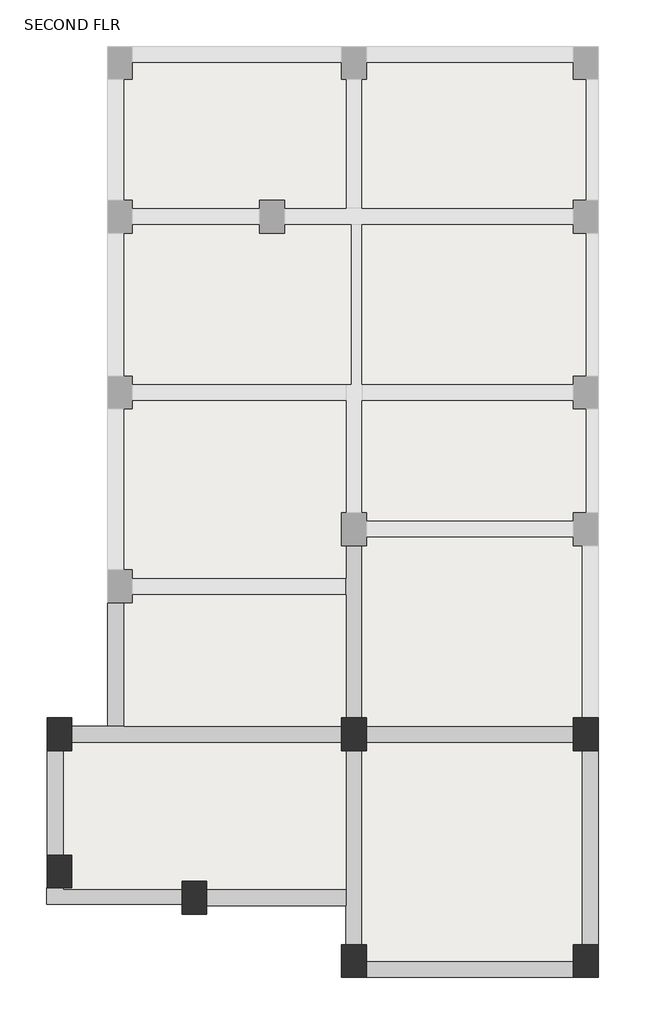
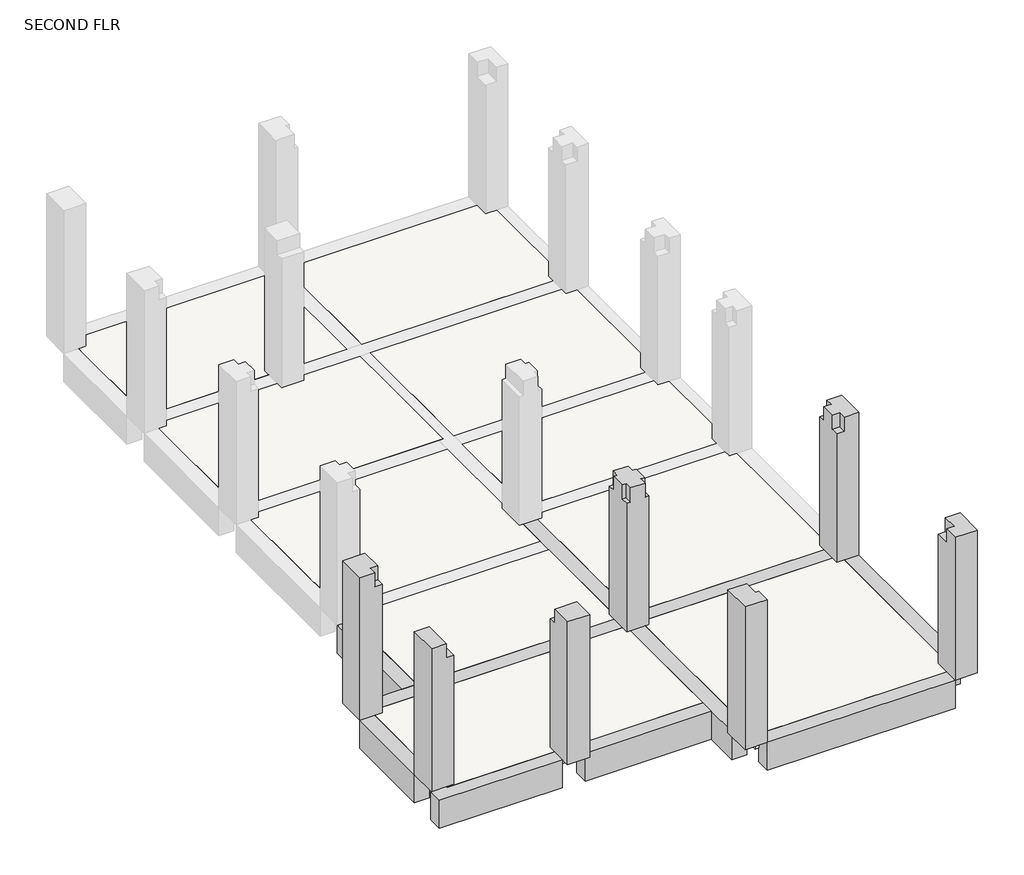
# One storey, part 1 of 2: 10 beams, 10 slabs, 7 columns.
"""IFC4 building model written with IfcOpenShell, lengths in millimetres."""

from ifc_helpers import new_model, si_unit, frame, origin, place, context, project, spatial, polyline, outline, extrude, faceted_brep, element, save

model = new_model("IFC4")

# Units and contexts
model_context = context("Model", 3, world=origin())
ifc_project = project(units=[si_unit("LENGTHUNIT", "METRE", prefix="MILLI")], contexts=[model_context])

# Site, building, storey
site = spatial("IfcSite", under=ifc_project)
building = spatial("IfcBuilding", under=site)
storey = spatial("IfcBuildingStorey", under=building, Name="SECOND FLR", Elevation=6048.0)

# Beams
placement = place(None, origin())
element("IfcBeam", 1, ObjectType="M_Concrete-Rectangular Beam : 300 x 600mm", at=placement, inside=storey, context=model_context, shape_type="SweptSolid", body=[
    extrude(outline(polyline([(2143.5134108, -6267.3380763), (2143.5134108, -6567.3380763), (-1646.635935, -6567.3380763), (-1646.635935, -6267.3380763), (2143.5134108, -6267.3380763)])), frame((0.0, 0.0, 5448.0), z_axis=(0.0, 0.0, 1.0), x_axis=(1.0, 0.0, 0.0)), (0.0, 0.0, 1.0), 600.0),
])
element("IfcBeam", 2, ObjectType="M_Concrete-Rectangular Beam : 300 x 600mm", at=placement, inside=storey, context=model_context, shape_type="SweptSolid", body=[
    extrude(outline(polyline([(2293.5134108, -2423.3693625), (2593.5134108, -2423.3693625), (2593.5134108, -5967.3380763), (2293.5134108, -5967.3380763), (2293.5134108, -2423.3693625)])), frame((0.0, 0.0, 5448.0), z_axis=(0.0, 0.0, 1.0), x_axis=(1.0, 0.0, 0.0)), (0.0, 0.0, 1.0), 600.0),
])
element("IfcBeam", 3, ObjectType="M_Concrete-Rectangular Beam : 300 x 600mm", at=placement, inside=storey, context=model_context, shape_type="SweptSolid", body=[
    extrude(outline(polyline([(-1646.635935, -2273.3693625), (-1646.635935, -1973.3693625), (2143.5134108, -1973.3693625), (2143.5134108, -2273.3693625), (-1646.635935, -2273.3693625)])), frame((0.0, 0.0, 5448.0), z_axis=(0.0, 0.0, 1.0), x_axis=(1.0, 0.0, 0.0)), (0.0, 0.0, 1.0), 600.0),
])
element("IfcBeam", 4, ObjectType="M_Concrete-Rectangular Beam : 300 x 600mm", at=placement, inside=storey, context=model_context, shape_type="Brep", body=[
    faceted_brep([(-1721.635935, -2423.3693625, 6048.0), (-2021.635935, -2423.3693625, 6048.0), (-2021.635935, -4959.2575036, 6048.0), (-2021.635935, -5259.2575036, 6048.0), (-2021.635935, -5967.3380763, 6048.0), (-1721.635935, -5967.3380763, 6048.0), (-1721.635935, -2423.3693625, 5448.0), (-1721.635935, -5967.3380763, 5448.0), (-2021.635935, -2423.3693625, 5448.0), (-2021.635935, -5967.3380763, 5448.0), (-2021.635935, -5259.2575036, 5448.0), (-2021.635935, -4959.2575036, 5448.0)], [[[0, 1, 2, 3, 4, 5]], [[6, 0, 5, 7]], [[8, 6, 7, 9, 10, 11]], [[1, 8, 11, 10, 9, 4, 3, 2]], [[1, 0, 6, 8]], [[4, 9, 7, 5]]]),
])
element("IfcBeam", 5, ObjectType="M_Concrete-Rectangular Beam : 300 x 600mm", at=placement, inside=storey, context=model_context, shape_type="Brep", body=[
    faceted_brep([(-1721.635935, 1328.1057379, 6048.0), (-2021.635935, 1328.1057379, 6048.0), (-2021.635935, 731.5941646, 6048.0), (-2021.635935, 431.5941646, 6048.0), (-2021.635935, -1823.3693625, 6048.0), (-1721.635935, -1823.3693625, 6048.0), (-1721.635935, 1328.1057379, 5448.0), (-1721.635935, -1823.3693625, 5448.0), (-2021.635935, 1328.1057379, 5448.0), (-2021.635935, -1823.3693625, 5448.0), (-2021.635935, 431.5941646, 5448.0), (-2021.635935, 731.5941646, 5448.0)], [[[0, 1, 2, 3, 4, 5]], [[6, 0, 5, 7]], [[8, 6, 7, 9, 10, 11]], [[1, 8, 11, 10, 9, 4, 3, 2]], [[1, 0, 6, 8]], [[4, 9, 7, 5]]]),
])
element("IfcBeam", 6, ObjectType="M_Concrete-Rectangular Beam : 300 x 600mm", at=placement, inside=storey, context=model_context, shape_type="Brep", body=[
    faceted_brep([(-4566.635935, -4959.2575036, 6048.0), (-4566.635935, -5259.2575036, 6048.0), (-2021.635935, -5259.2575036, 6048.0), (-2021.635935, -4959.2575036, 6048.0), (-4566.635935, -5259.2575036, 5448.0), (-2021.635935, -5259.2575036, 5448.0), (-4566.635935, -4959.2575036, 5448.0), (-2021.635935, -4959.2575036, 5448.0), (-2021.635935, -4959.2575036, 5748.0)], [[[0, 1, 2, 3]], [[1, 4, 5, 2]], [[4, 6, 7, 5]], [[6, 0, 3, 8, 7]], [[0, 6, 4, 1]], [[3, 2, 5, 7, 8]]]),
])
element("IfcBeam", 7, ObjectType="M_Concrete-Rectangular Beam : 300 x 600mm", at=placement, inside=storey, context=model_context, shape_type="Brep", body=[
    faceted_brep([(-7032.9642664, -1973.3693625, 6048.0), (-7032.9642664, -2273.3693625, 6048.0), (-2096.635935, -2273.3693625, 6048.0), (-2096.635935, -1973.3693625, 6048.0), (-6075.9642664, -1973.3693625, 6048.0), (-6375.9642664, -1973.3693625, 6048.0), (-7032.9642664, -1973.3693625, 5448.0), (-2096.635935, -1973.3693625, 5448.0), (-6075.9642664, -1973.3693625, 5448.0), (-6375.9642664, -1973.3693625, 5448.0), (-7032.9642664, -2273.3693625, 5448.0), (-2096.635935, -2273.3693625, 5448.0)], [[[0, 1, 2, 3, 4, 5]], [[6, 0, 5, 4, 3, 7, 8, 9]], [[10, 6, 9, 8, 7, 11]], [[1, 10, 11, 2]], [[2, 11, 7, 3]], [[1, 0, 6, 10]]]),
])
element("IfcBeam", 8, ObjectType="M_Concrete-Rectangular Beam : 300 x 600mm", at=placement, inside=storey, context=model_context, shape_type="Brep", body=[
    faceted_brep([(-6075.9642664, 281.5941646, 6048.0), (-6375.9642664, 281.5941646, 6048.0), (-6375.9642664, -1973.3693625, 6048.0), (-6075.9642664, -1973.3693625, 6048.0), (-6375.9642664, 281.5941646, 5448.0), (-6375.9642664, -1973.3693625, 5448.0), (-6075.9642664, 281.5941646, 5448.0), (-6075.9642664, -1973.3693625, 5448.0), (-6075.9642664, -1973.3693625, 5748.0)], [[[0, 1, 2, 3]], [[1, 4, 5, 2]], [[4, 6, 7, 5]], [[6, 0, 3, 8, 7]], [[0, 6, 4, 1]], [[3, 2, 5, 7, 8]]]),
])
element("IfcBeam", 9, ObjectType="M_Concrete-Rectangular Beam : 300 x 600mm", at=placement, inside=storey, context=model_context, shape_type="SweptSolid", body=[
    extrude(outline(polyline([(-7182.9642664, -4329.2575036), (-7482.9642664, -4329.2575036), (-7482.9642664, -2423.3693625), (-7182.9642664, -2423.3693625), (-7182.9642664, -4329.2575036)])), frame((0.0, 0.0, 5448.0), z_axis=(0.0, 0.0, 1.0), x_axis=(1.0, 0.0, 0.0)), (0.0, 0.0, 1.0), 600.0),
])
element("IfcBeam", 10, ObjectType="M_Concrete-Rectangular Beam : 300 x 600mm", at=placement, inside=storey, context=model_context, shape_type="Brep", body=[
    faceted_brep([(-7496.635935, -5229.2575036, 6048.0), (-7496.635935, -4929.2575036, 6048.0), (-7496.635935, -4929.2575036, 5448.0), (-7496.635935, -5229.2575036, 5448.0), (-5016.635935, -5229.2575036, 6048.0), (-5016.635935, -4959.2575036, 6048.0), (-7182.9642664, -4959.2575036, 6048.0), (-7182.9642664, -4929.2575036, 6048.0), (-7482.9642664, -4929.2575036, 6048.0), (-7182.9642664, -4929.2575036, 5748.0), (-7032.9642664, -4929.2575036, 5748.0), (-5016.635935, -4929.2575036, 5748.0), (-5016.635935, -4929.2575036, 5448.0), (-5016.635935, -5229.2575036, 5448.0), (-5016.635935, -4959.2575036, 5748.0), (-7182.9642664, -4959.2575036, 5748.0)], [[[0, 1, 2, 3]], [[1, 0, 4, 5, 6, 7, 8]], [[2, 1, 8, 7, 9, 10, 11, 12]], [[3, 2, 12, 13]], [[0, 3, 13, 4]], [[4, 13, 12, 11, 14, 5]], [[9, 15, 14, 11, 10]], [[15, 6, 5, 14]], [[6, 15, 9, 7]]]),
])

# Columns
element("IfcColumn", 11, ObjectType="M_Concrete-Rectangular-Column : 450 x 600mm", at=placement, inside=storey, context=model_context, shape_type="SweptSolid", body=[
    extrude(outline(polyline([(6048.0, -7482.9642664), (6048.0, -7032.9642664), (8796.0, -7032.9642664), (8796.0, -7182.9642664), (9096.0, -7182.9642664), (9096.0, -7482.9642664), (6048.0, -7482.9642664)])), frame((0.0, -4929.2575036, 0.0), z_axis=(0.0, 1.0, 0.0), x_axis=(0.0, 0.0, 1.0)), (0.0, 0.0, 1.0), 600.0),
])
element("IfcColumn", 12, ObjectType="M_Concrete-Rectangular-Column : 450 x 600mm", at=placement, inside=storey, context=model_context, shape_type="Brep", body=[
    faceted_brep([(-1646.635935, -1823.3693625, 6048.0), (-1646.635935, -2423.3693625, 6048.0), (-2096.635935, -2423.3693625, 6048.0), (-2096.635935, -1823.3693625, 6048.0), (-1646.635935, -1823.3693625, 8796.0), (-1646.635935, -1973.3693625, 8796.0), (-1646.635935, -1973.3693625, 9096.0), (-1646.635935, -2273.3693625, 9096.0), (-1646.635935, -2273.3693625, 8796.0), (-1646.635935, -2423.3693625, 8796.0), (-1721.635935, -2423.3693625, 8796.0), (-1721.635935, -2423.3693625, 9096.0), (-2021.635935, -2423.3693625, 9096.0), (-2021.635935, -2423.3693625, 8796.0), (-2096.635935, -2423.3693625, 8796.0), (-2096.635935, -2273.3693625, 8796.0), (-2096.635935, -2273.3693625, 9096.0), (-2096.635935, -1973.3693625, 9096.0), (-2096.635935, -1973.3693625, 8796.0), (-2096.635935, -1823.3693625, 8796.0), (-2021.635935, -1823.3693625, 8796.0), (-2021.635935, -1823.3693625, 9096.0), (-1721.635935, -1823.3693625, 9096.0), (-1721.635935, -1823.3693625, 8796.0), (-1721.635935, -1973.3693625, 9096.0), (-2021.635935, -1973.3693625, 9096.0), (-2021.635935, -2273.3693625, 9096.0), (-1721.635935, -2273.3693625, 9096.0), (-1721.635935, -1973.3693625, 8796.0), (-1721.635935, -2273.3693625, 8796.0), (-2021.635935, -1973.3693625, 8796.0), (-2021.635935, -2273.3693625, 8796.0)], [[[0, 1, 2, 3]], [[1, 0, 4, 5, 6, 7, 8, 9]], [[2, 1, 9, 10, 11, 12, 13, 14]], [[3, 2, 14, 15, 16, 17, 18, 19]], [[0, 3, 19, 20, 21, 22, 23, 4]], [[6, 24, 22, 21, 25, 17, 16, 26, 12, 11, 27, 7]], [[23, 28, 5, 4]], [[28, 24, 6, 5]], [[24, 28, 23, 22]], [[29, 10, 9, 8]], [[27, 29, 8, 7]], [[29, 27, 11, 10]], [[18, 30, 20, 19]], [[30, 25, 21, 20]], [[25, 30, 18, 17]], [[13, 31, 15, 14]], [[31, 26, 16, 15]], [[26, 31, 13, 12]]]),
])
element("IfcColumn", 13, ObjectType="M_Concrete-Rectangular-Column : 450 x 600mm", at=placement, inside=storey, context=model_context, shape_type="Brep", body=[
    faceted_brep([(-1646.635935, -5967.3380763, 6048.0), (-1646.635935, -6567.3380763, 6048.0), (-2096.635935, -6567.3380763, 6048.0), (-2096.635935, -5967.3380763, 6048.0), (-1646.635935, -5967.3380763, 8796.0), (-1646.635935, -6267.3380763, 8796.0), (-1646.635935, -6267.3380763, 9096.0), (-1646.635935, -6567.3380763, 9096.0), (-2096.635935, -6567.3380763, 9096.0), (-2096.635935, -5967.3380763, 9096.0), (-1721.635935, -5967.3380763, 9096.0), (-1721.635935, -5967.3380763, 8796.0), (-1721.635935, -6267.3380763, 9096.0), (-1721.635935, -6267.3380763, 8796.0)], [[[0, 1, 2, 3]], [[1, 0, 4, 5, 6, 7]], [[2, 1, 7, 8]], [[3, 2, 8, 9]], [[0, 3, 9, 10, 11, 4]], [[8, 7, 6, 12, 10, 9]], [[11, 13, 5, 4]], [[13, 12, 6, 5]], [[12, 13, 11, 10]]]),
])
element("IfcColumn", 14, ObjectType="M_Concrete-Rectangular-Column : 450 x 600mm", at=placement, inside=storey, context=model_context, shape_type="Brep", body=[
    faceted_brep([(2593.5134108, -1823.3693625, 6048.0), (2593.5134108, -2423.3693625, 6048.0), (2143.5134108, -2423.3693625, 6048.0), (2143.5134108, -1823.3693625, 6048.0), (2593.5134108, -1823.3693625, 9096.0), (2593.5134108, -2423.3693625, 9096.0), (2293.5134108, -2423.3693625, 9096.0), (2293.5134108, -2423.3693625, 8796.0), (2143.5134108, -2423.3693625, 8796.0), (2143.5134108, -2273.3693625, 8796.0), (2143.5134108, -2273.3693625, 9096.0), (2143.5134108, -1973.3693625, 9096.0), (2143.5134108, -1973.3693625, 8796.0), (2143.5134108, -1823.3693625, 8796.0), (2293.5134108, -1823.3693625, 8796.0), (2293.5134108, -1823.3693625, 9096.0), (2293.5134108, -1973.3693625, 9096.0), (2293.5134108, -2273.3693625, 9096.0), (2293.5134108, -1973.3693625, 8796.0), (2293.5134108, -2273.3693625, 8796.0)], [[[0, 1, 2, 3]], [[1, 0, 4, 5]], [[2, 1, 5, 6, 7, 8]], [[3, 2, 8, 9, 10, 11, 12, 13]], [[0, 3, 13, 14, 15, 4]], [[5, 4, 15, 16, 11, 10, 17, 6]], [[12, 18, 14, 13]], [[18, 16, 15, 14]], [[16, 18, 12, 11]], [[7, 19, 9, 8]], [[19, 17, 10, 9]], [[17, 19, 7, 6]]]),
])
element("IfcColumn", 15, ObjectType="M_Concrete-Rectangular-Column : 450 x 600mm", at=placement, inside=storey, context=model_context, shape_type="Brep", body=[
    faceted_brep([(2593.5134108, -5967.3380763, 6048.0), (2593.5134108, -6567.3380763, 6048.0), (2143.5134108, -6567.3380763, 6048.0), (2143.5134108, -5967.3380763, 6048.0), (2593.5134108, -5967.3380763, 9096.0), (2593.5134108, -6567.3380763, 9096.0), (2143.5134108, -6567.3380763, 9096.0), (2143.5134108, -6267.3380763, 9096.0), (2143.5134108, -6267.3380763, 8796.0), (2143.5134108, -5967.3380763, 8796.0), (2293.5134108, -5967.3380763, 8796.0), (2293.5134108, -5967.3380763, 9096.0), (2293.5134108, -6267.3380763, 9096.0), (2293.5134108, -6267.3380763, 8796.0)], [[[0, 1, 2, 3]], [[1, 0, 4, 5]], [[2, 1, 5, 6]], [[3, 2, 6, 7, 8, 9]], [[0, 3, 9, 10, 11, 4]], [[5, 4, 11, 12, 7, 6]], [[8, 13, 10, 9]], [[13, 12, 11, 10]], [[12, 13, 8, 7]]]),
])
element("IfcColumn", 16, ObjectType="M_Concrete-Rectangular-Column : 450 x 600mm", at=placement, inside=storey, context=model_context, shape_type="SweptSolid", body=[
    extrude(outline(polyline([(-4809.2575036, 6048.0), (-5409.2575036, 6048.0), (-5409.2575036, 9096.0), (-4959.2575036, 9096.0), (-4959.2575036, 8796.0), (-4809.2575036, 8796.0), (-4809.2575036, 6048.0)])), frame((-5016.635935, 0.0, 0.0), z_axis=(1.0, 0.0, 0.0), x_axis=(0.0, 1.0, 0.0)), (0.0, 0.0, 1.0), 450.0),
])
element("IfcColumn", 17, ObjectType="M_Concrete-Rectangular-Column : 450 x 600mm", at=placement, inside=storey, context=model_context, shape_type="Brep", body=[
    faceted_brep([(-7032.9642664, -1823.3693625, 6048.0), (-7032.9642664, -2423.3693625, 6048.0), (-7482.9642664, -2423.3693625, 6048.0), (-7482.9642664, -1823.3693625, 6048.0), (-7032.9642664, -1823.3693625, 9096.0), (-7032.9642664, -2273.3693625, 9096.0), (-7032.9642664, -2273.3693625, 8796.0), (-7032.9642664, -2423.3693625, 8796.0), (-7182.9642664, -2423.3693625, 8796.0), (-7182.9642664, -2423.3693625, 9096.0), (-7482.9642664, -2423.3693625, 9096.0), (-7482.9642664, -1823.3693625, 9096.0), (-7182.9642664, -2273.3693625, 9096.0), (-7182.9642664, -2273.3693625, 8796.0)], [[[0, 1, 2, 3]], [[1, 0, 4, 5, 6, 7]], [[2, 1, 7, 8, 9, 10]], [[3, 2, 10, 11]], [[0, 3, 11, 4]], [[11, 10, 9, 12, 5, 4]], [[13, 8, 7, 6]], [[12, 13, 6, 5]], [[13, 12, 9, 8]]]),
])

# Slabs
element("IfcSlab", 18, ObjectType="Generic 300mm", at=placement, inside=storey, context=model_context, shape_type="SweptSolid", body=[
    extrude(outline(polyline([(-2096.635935, 10150.0657956), (-2096.635935, 9850.0657956), (-2021.635935, 9850.0657956), (-2021.635935, 7491.506653), (-3146.635935, 7491.506653), (-3146.635935, 7641.506653), (-3596.635935, 7641.506653), (-3596.635935, 7491.506653), (-5925.9642664, 7491.506653), (-5925.9642664, 7641.506653), (-6075.9642664, 7641.506653), (-6075.9642664, 9850.0657956), (-5925.9642664, 9850.0657956), (-5925.9642664, 10150.0657956), (-2096.635935, 10150.0657956)])), frame((0.0, 0.0, 5748.0), z_axis=(0.0, 0.0, 1.0), x_axis=(1.0, 0.0, 0.0)), (0.0, 0.0, 1.0), 300.0),
])
element("IfcSlab", 19, ObjectType="Generic 300mm", at=placement, inside=storey, context=model_context, shape_type="Brep", body=[
    faceted_brep([(-1721.635935, 10150.0657956, 5748.0), (-1646.635935, 10150.0657956, 5748.0), (2143.5134108, 10150.0657956, 5748.0), (2368.5134108, 10150.0657956, 5748.0), (2368.5134108, 9850.0657956, 5748.0), (2368.5134108, 7641.506653, 5748.0), (2368.5134108, 7491.506653, 5748.0), (2143.5134108, 7491.506653, 5748.0), (-1721.635935, 7491.506653, 5748.0), (-1721.635935, 9850.0657956, 5748.0), (-1721.635935, 10150.0657956, 6048.0), (-1721.635935, 9850.0657956, 6048.0), (-1721.635935, 7491.506653, 6048.0), (2143.5134108, 7491.506653, 6048.0), (2368.5134108, 7491.506653, 6048.0), (2368.5134108, 7641.506653, 6048.0), (2368.5134108, 9850.0657956, 6048.0), (2368.5134108, 10150.0657956, 6048.0), (2143.5134108, 10150.0657956, 6048.0), (-1646.635935, 10150.0657956, 6048.0)], [[[0, 1, 2, 3, 4, 5, 6, 7, 8, 9]], [[10, 11, 12, 13, 14, 15, 16, 17, 18, 19]], [[3, 2, 1, 0, 10, 19, 18, 17]], [[6, 5, 4, 3, 17, 16, 15, 14]], [[8, 7, 6, 14, 13, 12]], [[0, 9, 8, 12, 11, 10]]]),
])
element("IfcSlab", 20, ObjectType="Generic 300mm", at=placement, inside=storey, context=model_context, shape_type="Brep", body=[
    faceted_brep([(-1721.635935, 7191.506653, 5748.0), (2143.5134108, 7191.506653, 5748.0), (2368.5134108, 7191.506653, 5748.0), (2368.5134108, 7041.506653, 5748.0), (2368.5134108, 4424.5351605, 5748.0), (2368.5134108, 4274.5351605, 5748.0), (2143.5134108, 4274.5351605, 5748.0), (-1721.635935, 4274.5351605, 5748.0), (-1721.635935, 7191.506653, 6048.0), (-1721.635935, 4274.5351605, 6048.0), (2143.5134108, 4274.5351605, 6048.0), (2368.5134108, 4274.5351605, 6048.0), (2368.5134108, 4424.5351605, 6048.0), (2368.5134108, 7041.506653, 6048.0), (2368.5134108, 7191.506653, 6048.0), (2143.5134108, 7191.506653, 6048.0)], [[[0, 1, 2, 3, 4, 5, 6, 7]], [[8, 9, 10, 11, 12, 13, 14, 15]], [[2, 1, 0, 8, 15, 14]], [[5, 4, 3, 2, 14, 13, 12, 11]], [[7, 6, 5, 11, 10, 9]], [[0, 7, 9, 8]]]),
])
element("IfcSlab", 21, ObjectType="Generic 300mm", at=placement, inside=storey, context=model_context, shape_type="Brep", body=[
    faceted_brep([(-6075.9642664, 7191.506653, 5748.0), (-5925.9642664, 7191.506653, 5748.0), (-3596.635935, 7191.506653, 5748.0), (-3146.635935, 7191.506653, 5748.0), (-2021.635935, 7191.506653, 5748.0), (-1928.7254278, 7191.506653, 5748.0), (-1928.7254278, 4274.5351605, 5748.0), (-2021.635935, 4274.5351605, 5748.0), (-5925.9642664, 4274.5351605, 5748.0), (-6075.9642664, 4274.5351605, 5748.0), (-6075.9642664, 4424.5351605, 5748.0), (-6075.9642664, 7041.506653, 5748.0), (-6075.9642664, 7191.506653, 6048.0), (-6075.9642664, 7041.506653, 6048.0), (-6075.9642664, 4424.5351605, 6048.0), (-6075.9642664, 4274.5351605, 6048.0), (-5925.9642664, 4274.5351605, 6048.0), (-2021.635935, 4274.5351605, 6048.0), (-1928.7254278, 4274.5351605, 6048.0), (-1928.7254278, 7191.506653, 6048.0), (-3146.635935, 7191.506653, 6048.0), (-3596.635935, 7191.506653, 6048.0), (-5925.9642664, 7191.506653, 6048.0)], [[[0, 1, 2, 3, 4, 5, 6, 7, 8, 9, 10, 11]], [[12, 13, 14, 15, 16, 17, 18, 19, 20, 21, 22]], [[5, 4, 3, 2, 1, 0, 12, 22, 21, 20, 19]], [[6, 5, 19, 18]], [[9, 8, 7, 6, 18, 17, 16, 15]], [[0, 11, 10, 9, 15, 14, 13, 12]]]),
])
element("IfcSlab", 22, ObjectType="Generic 300mm", at=placement, inside=storey, context=model_context, shape_type="Brep", body=[
    faceted_brep([(-1721.635935, 3974.5351605, 5748.0), (2143.5134108, 3974.5351605, 5748.0), (2368.5134108, 3974.5351605, 5748.0), (2368.5134108, 3824.5351605, 5748.0), (2368.5134108, 1928.1057379, 5748.0), (2368.5134108, 1778.1057379, 5748.0), (2143.5134108, 1778.1057379, 5748.0), (-1646.635935, 1778.1057379, 5748.0), (-1721.635935, 1778.1057379, 5748.0), (-1721.635935, 1928.1057379, 5748.0), (-1721.635935, 3974.5351605, 6048.0), (-1721.635935, 1928.1057379, 6048.0), (-1721.635935, 1778.1057379, 6048.0), (-1646.635935, 1778.1057379, 6048.0), (2143.5134108, 1778.1057379, 6048.0), (2368.5134108, 1778.1057379, 6048.0), (2368.5134108, 1928.1057379, 6048.0), (2368.5134108, 3824.5351605, 6048.0), (2368.5134108, 3974.5351605, 6048.0), (2143.5134108, 3974.5351605, 6048.0)], [[[0, 1, 2, 3, 4, 5, 6, 7, 8, 9]], [[10, 11, 12, 13, 14, 15, 16, 17, 18, 19]], [[2, 1, 0, 10, 19, 18]], [[5, 4, 3, 2, 18, 17, 16, 15]], [[8, 7, 6, 5, 15, 14, 13, 12]], [[0, 9, 8, 12, 11, 10]]]),
])
element("IfcSlab", 23, ObjectType="Generic 300mm", at=placement, inside=storey, context=model_context, shape_type="Brep", body=[
    faceted_brep([(-1721.635935, 1478.1057379, 5748.0), (-1646.635935, 1478.1057379, 5748.0), (2143.5134108, 1478.1057379, 5748.0), (2293.5134108, 1478.1057379, 5748.0), (2293.5134108, 1328.1057379, 5748.0), (2293.5134108, -1823.3693625, 5748.0), (2293.5134108, -1973.3693625, 5748.0), (2143.5134108, -1973.3693625, 5748.0), (-1646.635935, -1973.3693625, 5748.0), (-1721.635935, -1973.3693625, 5748.0), (-1721.635935, -1823.3693625, 5748.0), (-1721.635935, 1328.1057379, 5748.0), (-1721.635935, 1478.1057379, 6048.0), (-1721.635935, 1328.1057379, 6048.0), (-1721.635935, -1823.3693625, 6048.0), (-1721.635935, -1973.3693625, 6048.0), (-1646.635935, -1973.3693625, 6048.0), (2143.5134108, -1973.3693625, 6048.0), (2293.5134108, -1973.3693625, 6048.0), (2293.5134108, -1823.3693625, 6048.0), (2293.5134108, 1328.1057379, 6048.0), (2293.5134108, 1478.1057379, 6048.0), (2143.5134108, 1478.1057379, 6048.0), (-1646.635935, 1478.1057379, 6048.0)], [[[0, 1, 2, 3, 4, 5, 6, 7, 8, 9, 10, 11]], [[12, 13, 14, 15, 16, 17, 18, 19, 20, 21, 22, 23]], [[3, 2, 1, 0, 12, 23, 22, 21]], [[6, 5, 4, 3, 21, 20, 19, 18]], [[9, 8, 7, 6, 18, 17, 16, 15]], [[0, 11, 10, 9, 15, 14, 13, 12]]]),
])
element("IfcSlab", 24, ObjectType="Generic 300mm", at=placement, inside=storey, context=model_context, shape_type="Brep", body=[
    faceted_brep([(-1721.635935, -2273.3693625, 5748.0), (-1646.635935, -2273.3693625, 5748.0), (2143.5134108, -2273.3693625, 5748.0), (2293.5134108, -2273.3693625, 5748.0), (2293.5134108, -2423.3693625, 5748.0), (2293.5134108, -5967.3380763, 5748.0), (2293.5134108, -6267.3380763, 5748.0), (2143.5134108, -6267.3380763, 5748.0), (-1646.635935, -6267.3380763, 5748.0), (-1721.635935, -6267.3380763, 5748.0), (-1721.635935, -5967.3380763, 5748.0), (-1721.635935, -2423.3693625, 5748.0), (-1721.635935, -2273.3693625, 6048.0), (-1721.635935, -2423.3693625, 6048.0), (-1721.635935, -5967.3380763, 6048.0), (-1721.635935, -6267.3380763, 6048.0), (-1646.635935, -6267.3380763, 6048.0), (2143.5134108, -6267.3380763, 6048.0), (2293.5134108, -6267.3380763, 6048.0), (2293.5134108, -5967.3380763, 6048.0), (2293.5134108, -2423.3693625, 6048.0), (2293.5134108, -2273.3693625, 6048.0), (2143.5134108, -2273.3693625, 6048.0), (-1646.635935, -2273.3693625, 6048.0)], [[[0, 1, 2, 3, 4, 5, 6, 7, 8, 9, 10, 11]], [[12, 13, 14, 15, 16, 17, 18, 19, 20, 21, 22, 23]], [[3, 2, 1, 0, 12, 23, 22, 21]], [[6, 5, 4, 3, 21, 20, 19, 18]], [[9, 8, 7, 6, 18, 17, 16, 15]], [[0, 11, 10, 9, 15, 14, 13, 12]]]),
])
element("IfcSlab", 25, ObjectType="Generic 300mm", at=placement, inside=storey, context=model_context, shape_type="Brep", body=[
    faceted_brep([(-6075.9642664, 3974.5351605, 5748.0), (-5925.9642664, 3974.5351605, 5748.0), (-2021.635935, 3974.5351605, 5748.0), (-2021.635935, 1928.1057379, 5748.0), (-2021.635935, 1328.1057379, 5748.0), (-2021.635935, 731.5941646, 5748.0), (-5925.9642664, 731.5941646, 5748.0), (-6075.9642664, 731.5941646, 5748.0), (-6075.9642664, 881.5941646, 5748.0), (-6075.9642664, 3824.5351605, 5748.0), (-6075.9642664, 3974.5351605, 6048.0), (-6075.9642664, 3824.5351605, 6048.0), (-6075.9642664, 881.5941646, 6048.0), (-6075.9642664, 731.5941646, 6048.0), (-5925.9642664, 731.5941646, 6048.0), (-2021.635935, 731.5941646, 6048.0), (-2021.635935, 1328.1057379, 6048.0), (-2021.635935, 1928.1057379, 6048.0), (-2021.635935, 3974.5351605, 6048.0), (-5925.9642664, 3974.5351605, 6048.0)], [[[0, 1, 2, 3, 4, 5, 6, 7, 8, 9]], [[10, 11, 12, 13, 14, 15, 16, 17, 18, 19]], [[2, 1, 0, 10, 19, 18]], [[5, 4, 3, 2, 18, 17, 16, 15]], [[7, 6, 5, 15, 14, 13]], [[0, 9, 8, 7, 13, 12, 11, 10]]]),
])
element("IfcSlab", 26, ObjectType="Generic 300mm", at=placement, inside=storey, context=model_context, shape_type="Brep", body=[
    faceted_brep([(-6075.9642664, 431.5941646, 5748.0), (-5925.9642664, 431.5941646, 5748.0), (-2021.635935, 431.5941646, 5748.0), (-2021.635935, -1823.3693625, 5748.0), (-2021.635935, -1973.3693625, 5748.0), (-2096.635935, -1973.3693625, 5748.0), (-6075.9642664, -1973.3693625, 5748.0), (-6075.9642664, 281.5941646, 5748.0), (-6075.9642664, 431.5941646, 6048.0), (-6075.9642664, 281.5941646, 6048.0), (-6075.9642664, -1973.3693625, 6048.0), (-2096.635935, -1973.3693625, 6048.0), (-2021.635935, -1973.3693625, 6048.0), (-2021.635935, -1823.3693625, 6048.0), (-2021.635935, 431.5941646, 6048.0), (-5925.9642664, 431.5941646, 6048.0)], [[[0, 1, 2, 3, 4, 5, 6, 7]], [[8, 9, 10, 11, 12, 13, 14, 15]], [[2, 1, 0, 8, 15, 14]], [[4, 3, 2, 14, 13, 12]], [[6, 5, 4, 12, 11, 10]], [[0, 7, 6, 10, 9, 8]]]),
])
element("IfcSlab", 27, ObjectType="Generic 300mm", at=placement, inside=storey, context=model_context, shape_type="Brep", body=[
    faceted_brep([(-7182.9642664, -2273.3693625, 5748.0), (-7032.9642664, -2273.3693625, 5748.0), (-2096.635935, -2273.3693625, 5748.0), (-2021.635935, -2273.3693625, 5748.0), (-2021.635935, -2423.3693625, 5748.0), (-2021.635935, -4959.2575036, 5748.0), (-4566.635935, -4959.2575036, 5748.0), (-5016.635935, -4959.2575036, 5748.0), (-7182.9642664, -4959.2575036, 5748.0), (-7182.9642664, -4929.2575036, 5748.0), (-7182.9642664, -4329.2575036, 5748.0), (-7182.9642664, -2423.3693625, 5748.0), (-7182.9642664, -2273.3693625, 6048.0), (-7182.9642664, -2423.3693625, 6048.0), (-7182.9642664, -4329.2575036, 6048.0), (-7182.9642664, -4929.2575036, 6048.0), (-7182.9642664, -4959.2575036, 6048.0), (-5016.635935, -4959.2575036, 6048.0), (-4566.635935, -4959.2575036, 6048.0), (-2021.635935, -4959.2575036, 6048.0), (-2021.635935, -2423.3693625, 6048.0), (-2021.635935, -2273.3693625, 6048.0), (-2096.635935, -2273.3693625, 6048.0), (-7032.9642664, -2273.3693625, 6048.0)], [[[0, 1, 2, 3, 4, 5, 6, 7, 8, 9, 10, 11]], [[12, 13, 14, 15, 16, 17, 18, 19, 20, 21, 22, 23]], [[3, 2, 1, 0, 12, 23, 22, 21]], [[5, 4, 3, 21, 20, 19]], [[8, 7, 6, 5, 19, 18, 17, 16]], [[0, 11, 10, 9, 8, 16, 15, 14, 13, 12]]]),
])

save(model, "model.ifc")

# Revit data of these elements
# Type "M_Concrete-Rectangular Beam : 300 x 600mm"
#   Length [instance default] = 1524 mm
#   b = 300 mm
#   h = 600 mm
#   Structural Material [instance default] = Concrete, Cast-in-Place gray
#   Assembly Code = ""
# Type "M_Concrete-Rectangular-Column : 450 x 600mm"
#   b = 450 mm
#   h = 600 mm
#   Structural Material [instance default] = Concrete, Cast-in-Place gray
# Type "Generic 300mm"
#   Function = 0
#   Layers, outside or top first: 300 mm no material (function 1)
# Elements 1, 2, 3, 4, 5, 6, 7, 8, 9, 10 (IfcBeam, "M_Concrete-Rectangular Beam : 300 x 600mm")
#   Structural Material = Concrete, Cast-in-Place gray
#   Phase Created = New Construction
#   Materials on its faces: "Concrete, Cast-in-Place gray"
# Elements 11, 12, 13, 14, 15, 16, 17 (IfcColumn, "M_Concrete-Rectangular-Column : 450 x 600mm")
#   Structural Material = Concrete, Cast-in-Place gray
#   Phase Created = New Construction
#   Materials on its faces: "Concrete, Cast-in-Place gray"
# Element 18 (IfcSlab, "Generic 300mm")
#   Height Offset From Level = 0 mm
#   built-in parameter 1001954 = 1
#   Phase Created = New Construction
#   Materials on its faces: "Default Floor"
# Elements 19, 20, 21, 22, 23, 24, 25, 26, 27 (IfcSlab, "Generic 300mm")
#   built-in parameter 1001955 = 3.14159 (stored number, unit not read)
#   Height Offset From Level = 0 mm
#   built-in parameter 1001954 = 1
#   Phase Created = New Construction
#   Materials on its faces: "Default Floor"
# Materials
#   "Concrete, Cast-in-Place gray": class "Concrete", colour RGB 192 192 192, transparency 0, Description = "Cast-in-place concrete", Cost = 0
#   "Default Floor": colour RGB 127 127 127, transparency 0, Cost = 0
